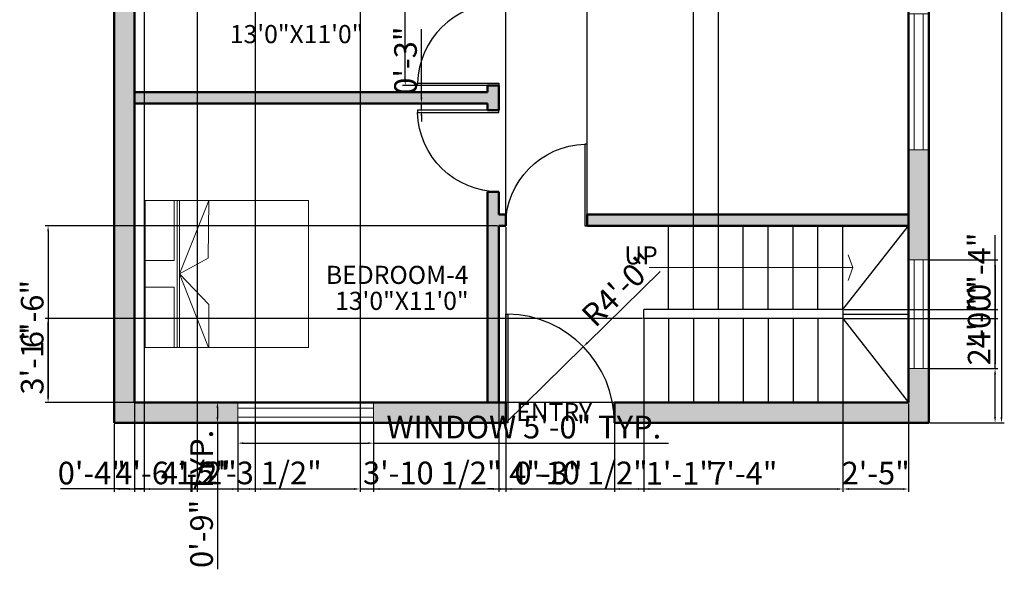
# Model space of a CAD drawing. Units: inches. Extents: x 2719 to 3167, y 1639 to 2327.
# Tile 1 of 4: x 2727 to 3162, y 1639 to 1881. Entities that reach past the tile are written whole.
import ezdxf

# ---------------------------------------------------------------- set-up
doc = ezdxf.new("R2010")
doc.units = ezdxf.units.IN
for name, color, linetype, lineweight in [('A-ANNO-DIMS', 121, 'Continuous', 18), ('A-ANNO-SYMB', 7, 'Continuous', 18), ('A-ANNO-TEXT', 121, 'Continuous', 18), ('A-AREA-IDEN', 121, 'Continuous', 18), ('A-DOOR', 50, 'Continuous', 25), ('A-FLOR-STRS', 7, 'Continuous', 25), ('A-FURN', 211, 'Continuous', 18), ('A-GLAZ', 191, 'Continuous', 18), ('A-WALL', 7, 'Continuous', 50)]:
    doc.layers.add(name, color=color, linetype=linetype, lineweight=lineweight)
doc.layers.add('A-WALL-PATT', color=251, linetype='Continuous', lineweight=13, true_color=0x636466)
doc.styles.get("Standard").update_dxf_attribs({"font": 'arial.ttf'})
doc.dimstyles.new('ISO-25', dxfattribs={"dimtxt": 10, "dimasz": 2.5, "dimexe": 1.25, "dimexo": 0.625, "dimtad": 1, "dimdec": 0, "dimlunit": 3, "dimtxsty": 'Standard', "dimcen": 2.5, "dimadec": 0, "dimazin": 0, "dimtfac": 1, "dimtdec": 0, "dimtmove": 0, "dimatfit": 3, "dimfxl": 1, "dimarcsym": 0})

# ---------------------------------------------------------------- blocks, each defined once
blk = doc.blocks.new('*D2')
at = {"layer": 'A-ANNO-DIMS', "color": 0, "lineweight": -2, "transparency": 16777216}
for p, q in [((3129.42, 2243.44), (3162.14, 2243.44)), ((3160.89, 2240.94), (3160.89, 1705.94)), ((3129.42, 1703.44), (3162.14, 1703.44))]:
    blk.add_line(p, q, dxfattribs=at)
at = {"layer": 'A-ANNO-DIMS', "color": 0, "transparency": 16777216}
for points in [[(3160.47, 2240.94), (3161.31, 2240.94), (3160.89, 2243.44)], [(3160.47, 1705.94), (3161.31, 1705.94), (3160.89, 1703.44)]]:
    blk.add_solid(points, dxfattribs=at)
at = {"layer": 'Defpoints', "color": 0, "transparency": 16777216}
for p in [(3128.8, 2243.44), (3128.8, 1703.44), (3160.89, 1703.44)]:
    blk.add_point(p, dxfattribs=at)
at = {"layer": 'A-ANNO-DIMS', "color": 0, "transparency": 16777216, "insert": (3155.18, 1973.44), "char_height": 10, "attachment_point": 5, "rotation": 90}
blk.add_mtext("45'", dxfattribs=at)
blk = doc.blocks.new('BED-DOUBLE')
for p, q in [((0, 57.96), (64.91, 57.96)), ((0, 56.96), (64.91, 56.96)), ((32.46, 56.96), (0, 44.1)), ((32.46, 56.96), (18.94, 44.05)), ((32.46, 56.96), (64.91, 44.04)), ((32.46, 56.96), (39.4, 44.29)), ((18.94, 44.05), (0, 44.05)), ((39.4, 44.29), (64.91, 44.04))]:
    blk.add_line(p, q)
for points in [[(0, 72.15), (64.91, 72.15), (64.91, 0), (0, 0)], [(0, 72.15), (26.55, 72.15), (26.55, 59.27), (0, 59.27)], [(38.37, 72.15), (64.91, 72.15), (64.91, 59.27), (38.37, 59.27)]]:
    blk.add_lwpolyline(points, close=True)
blk = doc.blocks.new('WIN-60IN')
for p, q in [((9, 60), (0, 60)), ((2.5, 60), (2.5, 0)), ((6.5, 60), (6.5, 0)), ((9, 0), (0, 0))]:
    blk.add_line(p, q)
blk = doc.blocks.new('DOOR-36IN-SWING')
for p, q in [((0, 0), (0, 1)), ((0, 1), (36, 1)), ((36, 0), (0, 0)), ((36, 1), (36, 0))]:
    blk.add_line(p, q)
blk.add_arc((35.99, 0), 36, 89.9779, 178.4083)
blk = doc.blocks.new('*D7')
at = {"layer": 'A-ANNO-DIMS', "color": 0, "lineweight": -2, "transparency": 16777216}
for p, q in [((2823.4, 1702.81), (2823.4, 1693.19)), ((2883.4, 1702.81), (2883.4, 1693.19)), ((2825.9, 1694.44), (2880.9, 1694.44)), ((2883.4, 1694.44), (3013.69, 1694.44))]:
    blk.add_line(p, q, dxfattribs=at)
at = {"layer": 'A-ANNO-DIMS', "color": 0, "transparency": 16777216}
for points in [[(2825.9, 1694.85), (2825.9, 1694.02), (2823.4, 1694.44)], [(2880.9, 1694.85), (2880.9, 1694.02), (2883.4, 1694.44)]]:
    blk.add_solid(points, dxfattribs=at)
at = {"layer": 'Defpoints', "color": 0, "transparency": 16777216}
for p in [(2823.4, 1703.44), (2883.4, 1703.44), (2883.4, 1694.44)]:
    blk.add_point(p, dxfattribs=at)
at = {"layer": 'A-ANNO-DIMS', "color": 0, "transparency": 16777216, "insert": (2949.79, 1700.24), "char_height": 10, "attachment_point": 5}
blk.add_mtext('WINDOW 5\'-0" TYP.', dxfattribs=at)
blk = doc.blocks.new('*D8')
at = {"layer": 'A-ANNO-DIMS', "color": 0, "lineweight": -2, "transparency": 16777216}
for p, q in [((2822.77, 1712.44), (2813.15, 1712.44)), ((2814.4, 1709.94), (2814.4, 1705.94)), ((2822.77, 1703.44), (2813.15, 1703.44)), ((2814.4, 1703.44), (2814.4, 1638.73))]:
    blk.add_line(p, q, dxfattribs=at)
at = {"layer": 'A-ANNO-DIMS', "color": 0, "transparency": 16777216}
for points in [[(2813.98, 1709.94), (2814.82, 1709.94), (2814.4, 1712.44)], [(2813.98, 1705.94), (2814.82, 1705.94), (2814.4, 1703.44)]]:
    blk.add_solid(points, dxfattribs=at)
at = {"layer": 'Defpoints', "color": 0, "transparency": 16777216}
for p in [(2823.4, 1712.44), (2814.4, 1703.44), (2823.4, 1703.44)]:
    blk.add_point(p, dxfattribs=at)
at = {"layer": 'A-ANNO-DIMS', "color": 0, "transparency": 16777216, "insert": (2808.67, 1669.83), "char_height": 10, "attachment_point": 5, "rotation": 90}
blk.add_mtext('0\'-9" TYP.', dxfattribs=at)
blk = doc.blocks.new('*D11')
at = {"layer": 'A-ANNO-DIMS', "color": 0, "lineweight": -2, "transparency": 16777216}
for p, q in [((2897.39, 1888.44), (2897.39, 2011.64)), ((2902.17, 1888.44), (2896.14, 1888.44)), ((2897.39, 1854.94), (2897.39, 1885.94)), ((2902.17, 1852.44), (2896.14, 1852.44))]:
    blk.add_line(p, q, dxfattribs=at)
at = {"layer": 'A-ANNO-DIMS', "color": 0, "transparency": 16777216}
for points in [[(2896.98, 1885.94), (2897.81, 1885.94), (2897.39, 1888.44)], [(2896.98, 1854.94), (2897.81, 1854.94), (2897.39, 1852.44)]]:
    blk.add_solid(points, dxfattribs=at)
at = {"layer": 'Defpoints', "color": 0, "transparency": 16777216}
for p in [(2897.39, 1888.44), (2902.8, 1888.44), (2902.8, 1852.44)]:
    blk.add_point(p, dxfattribs=at)
at = {"layer": 'A-ANNO-DIMS', "color": 0, "transparency": 16777216, "insert": (2891.59, 1951.29), "char_height": 10, "attachment_point": 5, "rotation": 90}
blk.add_mtext('DOOR A 3\'-0" TYP.', dxfattribs=at)
blk = doc.blocks.new('*D15')
at = {"layer": 'A-ANNO-DIMS', "color": 0, "lineweight": -2, "transparency": 16777216}
for p, q in [((2768.8, 1702.81), (2768.8, 1672.94)), ((2823.4, 1702.81), (2823.4, 1672.94)), ((2771.3, 1674.19), (2820.9, 1674.19))]:
    blk.add_line(p, q, dxfattribs=at)
at = {"layer": 'A-ANNO-DIMS', "color": 0, "transparency": 16777216}
for points in [[(2771.3, 1674.6), (2771.3, 1673.77), (2768.8, 1674.19)], [(2820.9, 1674.6), (2820.9, 1673.77), (2823.4, 1674.19)]]:
    blk.add_solid(points, dxfattribs=at)
at = {"layer": 'Defpoints', "color": 0, "transparency": 16777216}
for p in [(2768.8, 1703.44), (2823.4, 1703.44), (2823.4, 1674.19)]:
    blk.add_point(p, dxfattribs=at)
at = {"layer": 'A-ANNO-DIMS', "color": 0, "transparency": 16777216, "insert": (2796.1, 1679.98), "char_height": 10, "attachment_point": 5}
blk.add_mtext('4\'-6 1/2"', dxfattribs=at)
blk = doc.blocks.new('*D16')
at = {"layer": 'A-ANNO-DIMS', "color": 0, "lineweight": -2, "transparency": 16777216}
for p, q in [((2883.4, 1702.81), (2883.4, 1672.94)), ((2941.8, 1702.81), (2941.8, 1672.94)), ((2885.9, 1674.19), (2939.3, 1674.19)), ((2941.8, 1674.19), (3003.6, 1674.19))]:
    blk.add_line(p, q, dxfattribs=at)
at = {"layer": 'A-ANNO-DIMS', "color": 0, "transparency": 16777216}
for points in [[(2885.9, 1674.6), (2885.9, 1673.77), (2883.4, 1674.19)], [(2939.3, 1674.6), (2939.3, 1673.77), (2941.8, 1674.19)]]:
    blk.add_solid(points, dxfattribs=at)
at = {"layer": 'Defpoints', "color": 0, "transparency": 16777216}
for p in [(2883.4, 1703.44), (2941.8, 1703.44), (2941.8, 1674.19)]:
    blk.add_point(p, dxfattribs=at)
at = {"layer": 'A-ANNO-DIMS', "color": 0, "transparency": 16777216, "insert": (2973.95, 1679.98), "char_height": 10, "attachment_point": 5}
blk.add_mtext('4\'-10 1/2"', dxfattribs=at)
blk = doc.blocks.new('*D26')
at = {"layer": 'A-ANNO-DIMS', "color": 0, "lineweight": -2, "transparency": 16777216}
for p, q in [((3158.05, 1727.34), (3158.05, 1757.84)), ((3129.42, 1727.34), (3159.3, 1727.34)), ((3158.05, 1705.94), (3158.05, 1724.84)), ((3129.42, 1703.44), (3159.3, 1703.44))]:
    blk.add_line(p, q, dxfattribs=at)
at = {"layer": 'A-ANNO-DIMS', "color": 0, "transparency": 16777216}
for points in [[(3157.63, 1724.84), (3158.46, 1724.84), (3158.05, 1727.34)], [(3157.63, 1705.94), (3158.46, 1705.94), (3158.05, 1703.44)]]:
    blk.add_solid(points, dxfattribs=at)
at = {"layer": 'Defpoints', "color": 0, "transparency": 16777216}
for p in [(3128.8, 1727.34), (3158.05, 1727.34), (3128.8, 1703.44)]:
    blk.add_point(p, dxfattribs=at)
at = {"layer": 'A-ANNO-DIMS', "color": 0, "transparency": 16777216, "insert": (3152.32, 1743.84), "char_height": 10, "attachment_point": 5, "rotation": 90}
blk.add_mtext('2\'-0"', dxfattribs=at)
blk = doc.blocks.new('*D27')
at = {"layer": 'A-ANNO-DIMS', "color": 0, "lineweight": -2, "transparency": 16777216}
for p, q in [((3129.42, 1775.34), (3159.3, 1775.34)), ((3158.05, 1772.84), (3158.05, 1729.84)), ((3129.42, 1727.34), (3159.3, 1727.34))]:
    blk.add_line(p, q, dxfattribs=at)
at = {"layer": 'A-ANNO-DIMS', "color": 0, "transparency": 16777216}
for points in [[(3157.63, 1772.84), (3158.46, 1772.84), (3158.05, 1775.34)], [(3157.63, 1729.84), (3158.46, 1729.84), (3158.05, 1727.34)]]:
    blk.add_solid(points, dxfattribs=at)
at = {"layer": 'Defpoints', "color": 0, "transparency": 16777216}
for p in [(3128.8, 1775.34), (3128.8, 1727.34), (3158.05, 1727.34)]:
    blk.add_point(p, dxfattribs=at)
at = {"layer": 'A-ANNO-DIMS', "color": 0, "transparency": 16777216, "insert": (3152.32, 1751.34), "char_height": 10, "attachment_point": 5, "rotation": 90}
blk.add_mtext('4\'-0"', dxfattribs=at)
blk = doc.blocks.new('*D31')
at = {"layer": 'A-ANNO-DIMS', "color": 0, "lineweight": -2, "transparency": 16777216}
for p, q in [((2777.8, 1985.81), (2777.8, 1672.94)), ((2805.5, 1985.81), (2805.5, 1672.94)), ((2780.3, 1674.19), (2803, 1674.19)), ((2805.5, 1674.19), (2859.31, 1674.19))]:
    blk.add_line(p, q, dxfattribs=at)
at = {"layer": 'A-ANNO-DIMS', "color": 0, "transparency": 16777216}
for points in [[(2780.3, 1674.6), (2780.3, 1673.77), (2777.8, 1674.19)], [(2803, 1674.6), (2803, 1673.77), (2805.5, 1674.19)]]:
    blk.add_solid(points, dxfattribs=at)
at = {"layer": 'Defpoints', "color": 0, "transparency": 16777216}
for p in [(2777.8, 1986.44), (2805.5, 1986.44), (2805.5, 1674.19)]:
    blk.add_point(p, dxfattribs=at)
at = {"layer": 'A-ANNO-DIMS', "color": 0, "transparency": 16777216, "insert": (2833.65, 1679.99), "char_height": 10, "attachment_point": 5}
blk.add_mtext('2\'-3 1/2"', dxfattribs=at)
blk = doc.blocks.new('*D36')
at = {"layer": 'A-ANNO-DIMS', "color": 0, "lineweight": -2, "transparency": 16777216}
for p, q in [((2782.04, 2006.33), (2782.04, 1672.94)), ((2777.8, 1985.81), (2777.8, 1672.94)), ((2775.3, 1674.19), (2744.96, 1674.19)), ((2782.04, 1674.19), (2777.8, 1674.19)), ((2784.54, 1674.19), (2787.04, 1674.19))]:
    blk.add_line(p, q, dxfattribs=at)
at = {"layer": 'A-ANNO-DIMS', "color": 0, "transparency": 16777216}
for points in [[(2775.3, 1674.6), (2775.3, 1673.77), (2777.8, 1674.19)], [(2784.54, 1674.6), (2784.54, 1673.77), (2782.04, 1674.19)]]:
    blk.add_solid(points, dxfattribs=at)
at = {"layer": 'Defpoints', "color": 0, "transparency": 16777216}
for p in [(2782.04, 2006.96), (2777.8, 1986.44), (2777.8, 1674.19)]:
    blk.add_point(p, dxfattribs=at)
at = {"layer": 'A-ANNO-DIMS', "color": 0, "transparency": 16777216, "insert": (2758.88, 1679.92), "char_height": 10, "attachment_point": 5}
blk.add_mtext('0\'-4"', dxfattribs=at)
blk = doc.blocks.new('*D37')
at = {"layer": 'A-ANNO-DIMS', "color": 0, "lineweight": -2, "transparency": 16777216}
for p, q in [((2831.04, 2061.64), (2831.04, 1672.94)), ((2877.4, 2061.64), (2877.4, 1672.94)), ((2833.54, 1674.19), (2874.9, 1674.19)), ((2877.4, 1674.19), (2938.79, 1674.19))]:
    blk.add_line(p, q, dxfattribs=at)
at = {"layer": 'A-ANNO-DIMS', "color": 0, "transparency": 16777216}
for points in [[(2833.54, 1674.6), (2833.54, 1673.77), (2831.04, 1674.19)], [(2874.9, 1674.6), (2874.9, 1673.77), (2877.4, 1674.19)]]:
    blk.add_solid(points, dxfattribs=at)
at = {"layer": 'Defpoints', "color": 0, "transparency": 16777216}
for p in [(2831.04, 2062.26), (2877.4, 2062.26), (2877.4, 1674.19)]:
    blk.add_point(p, dxfattribs=at)
at = {"layer": 'A-ANNO-DIMS', "color": 0, "transparency": 16777216, "insert": (2909.34, 1679.99), "char_height": 10, "attachment_point": 5}
blk.add_mtext('3\'-10 1/2"', dxfattribs=at)
blk = doc.blocks.new('*D39')
at = {"layer": 'A-ANNO-DIMS', "color": 0, "lineweight": -2, "transparency": 16777216}
for p, q in [((2777.8, 2084.81), (2777.8, 1672.94)), ((2831.04, 2061.64), (2831.04, 1672.94)), ((2780.3, 1674.19), (2828.54, 1674.19))]:
    blk.add_line(p, q, dxfattribs=at)
at = {"layer": 'A-ANNO-DIMS', "color": 0, "transparency": 16777216}
for points in [[(2780.3, 1674.6), (2780.3, 1673.77), (2777.8, 1674.19)], [(2828.54, 1674.6), (2828.54, 1673.77), (2831.04, 1674.19)]]:
    blk.add_solid(points, dxfattribs=at)
at = {"layer": 'Defpoints', "color": 0, "transparency": 16777216}
for p in [(2777.8, 2085.44), (2831.04, 2062.26), (2831.04, 1674.19)]:
    blk.add_point(p, dxfattribs=at)
at = {"layer": 'A-ANNO-DIMS', "color": 0, "transparency": 16777216, "insert": (2804.42, 1679.9), "char_height": 10, "attachment_point": 5}
blk.add_mtext('4\'-5"', dxfattribs=at)
blk = doc.blocks.new('*D41')
at = {"layer": 'A-ANNO-DIMS', "color": 0, "lineweight": -2, "transparency": 16777216}
for p, q in [((3002.8, 1711.81), (3002.8, 1672.94)), ((3090.8, 1711.81), (3090.8, 1672.94)), ((3005.3, 1674.19), (3088.3, 1674.19))]:
    blk.add_line(p, q, dxfattribs=at)
at = {"layer": 'A-ANNO-DIMS', "color": 0, "transparency": 16777216}
for points in [[(3005.3, 1674.6), (3005.3, 1673.77), (3002.8, 1674.19)], [(3088.3, 1674.6), (3088.3, 1673.77), (3090.8, 1674.19)]]:
    blk.add_solid(points, dxfattribs=at)
at = {"layer": 'Defpoints', "color": 0, "transparency": 16777216}
for p in [(3002.8, 1712.44), (3090.8, 1712.44), (3090.8, 1674.19)]:
    blk.add_point(p, dxfattribs=at)
at = {"layer": 'A-ANNO-DIMS', "color": 0, "transparency": 16777216, "insert": (3046.8, 1679.81), "char_height": 10, "attachment_point": 5}
blk.add_mtext('7\'-4"', dxfattribs=at)
blk = doc.blocks.new('*D42')
at = {"layer": 'A-ANNO-DIMS', "color": 0, "lineweight": -2, "transparency": 16777216}
for p, q in [((3090.8, 1711.81), (3090.8, 1672.94)), ((3119.8, 1711.81), (3119.8, 1672.94)), ((3093.3, 1674.19), (3117.3, 1674.19))]:
    blk.add_line(p, q, dxfattribs=at)
at = {"layer": 'A-ANNO-DIMS', "color": 0, "transparency": 16777216}
for points in [[(3093.3, 1674.6), (3093.3, 1673.77), (3090.8, 1674.19)], [(3117.3, 1674.6), (3117.3, 1673.77), (3119.8, 1674.19)]]:
    blk.add_solid(points, dxfattribs=at)
at = {"layer": 'Defpoints', "color": 0, "transparency": 16777216}
for p in [(3090.8, 1712.44), (3119.8, 1712.44), (3119.8, 1674.19)]:
    blk.add_point(p, dxfattribs=at)
at = {"layer": 'A-ANNO-DIMS', "color": 0, "transparency": 16777216, "insert": (3105.3, 1679.92), "char_height": 10, "attachment_point": 5}
blk.add_mtext('2\'-5"', dxfattribs=at)
blk = doc.blocks.new('*D43')
at = {"layer": 'A-ANNO-DIMS', "color": 0, "lineweight": -2, "transparency": 16777216}
for p, q in [((2989.8, 1711.81), (2989.8, 1672.94)), ((3002.8, 1711.81), (3002.8, 1672.94)), ((2992.3, 1674.19), (3000.3, 1674.19)), ((3002.8, 1674.19), (3032.19, 1674.19))]:
    blk.add_line(p, q, dxfattribs=at)
at = {"layer": 'A-ANNO-DIMS', "color": 0, "transparency": 16777216}
for points in [[(2992.3, 1674.6), (2992.3, 1673.77), (2989.8, 1674.19)], [(3000.3, 1674.6), (3000.3, 1673.77), (3002.8, 1674.19)]]:
    blk.add_solid(points, dxfattribs=at)
at = {"layer": 'Defpoints', "color": 0, "transparency": 16777216}
for p in [(2989.8, 1712.44), (3002.8, 1712.44), (3002.8, 1674.19)]:
    blk.add_point(p, dxfattribs=at)
at = {"layer": 'A-ANNO-DIMS', "color": 0, "transparency": 16777216, "insert": (3018.74, 1679.83), "char_height": 10, "attachment_point": 5}
blk.add_mtext('1\'-1"', dxfattribs=at)
blk = doc.blocks.new('*D44')
at = {"layer": 'A-ANNO-DIMS', "color": 0, "lineweight": -2, "transparency": 16777216}
for p, q in [((3002.17, 1749.44), (2738.3, 1749.44)), ((2739.55, 1714.94), (2739.55, 1746.94)), ((3002.17, 1712.44), (2738.3, 1712.44))]:
    blk.add_line(p, q, dxfattribs=at)
at = {"layer": 'A-ANNO-DIMS', "color": 0, "transparency": 16777216}
for points in [[(2739.13, 1746.94), (2739.96, 1746.94), (2739.55, 1749.44)], [(2739.13, 1714.94), (2739.96, 1714.94), (2739.55, 1712.44)]]:
    blk.add_solid(points, dxfattribs=at)
at = {"layer": 'Defpoints', "color": 0, "transparency": 16777216}
for p in [(2739.55, 1749.44), (3002.8, 1749.44), (3002.8, 1712.44)]:
    blk.add_point(p, dxfattribs=at)
at = {"layer": 'A-ANNO-DIMS', "color": 0, "transparency": 16777216, "insert": (2733.81, 1730.94), "char_height": 10, "attachment_point": 5, "rotation": 90}
blk.add_mtext('3\'-1"', dxfattribs=at)
blk = doc.blocks.new('*D45')
at = {"layer": 'A-ANNO-DIMS', "color": 0, "lineweight": -2, "transparency": 16777216}
for p, q in [((3158.05, 1755.94), (3158.05, 1786.27)), ((3091.42, 1753.44), (3159.3, 1753.44)), ((3091.42, 1749.44), (3159.3, 1749.44)), ((3158.05, 1749.44), (3158.05, 1753.44)), ((3158.05, 1746.94), (3158.05, 1744.44))]:
    blk.add_line(p, q, dxfattribs=at)
at = {"layer": 'A-ANNO-DIMS', "color": 0, "transparency": 16777216}
for points in [[(3157.63, 1755.94), (3158.46, 1755.94), (3158.05, 1753.44)], [(3157.63, 1746.94), (3158.46, 1746.94), (3158.05, 1749.44)]]:
    blk.add_solid(points, dxfattribs=at)
at = {"layer": 'Defpoints', "color": 0, "transparency": 16777216}
for p in [(3090.8, 1753.44), (3090.8, 1749.44), (3158.05, 1753.44)]:
    blk.add_point(p, dxfattribs=at)
at = {"layer": 'A-ANNO-DIMS', "color": 0, "transparency": 16777216, "insert": (3152.32, 1772.35), "char_height": 10, "attachment_point": 5, "rotation": 90}
blk.add_mtext('0\'-4"', dxfattribs=at)
blk = doc.blocks.new('*D46')
at = {"layer": 'A-ANNO-DIMS', "color": 0, "lineweight": -2, "transparency": 16777216}
for p, q in [((3024.8, 1791.06), (3024.8, 2273.94)), ((3027.3, 2272.69), (3033.3, 2272.69)), ((3035.8, 1791.06), (3035.8, 2273.94)), ((3035.8, 2272.69), (3073.9, 2272.69))]:
    blk.add_line(p, q, dxfattribs=at)
at = {"layer": 'A-ANNO-DIMS', "color": 0, "transparency": 16777216}
for points in [[(3027.3, 2273.1), (3027.3, 2272.27), (3024.8, 2272.69)], [(3033.3, 2273.1), (3033.3, 2272.27), (3035.8, 2272.69)]]:
    blk.add_solid(points, dxfattribs=at)
at = {"layer": 'Defpoints', "color": 0, "transparency": 16777216}
for p in [(3035.8, 2272.69), (3024.8, 1790.44), (3035.8, 1790.44)]:
    blk.add_point(p, dxfattribs=at)
at = {"layer": 'A-ANNO-DIMS', "color": 0, "transparency": 16777216, "insert": (3056.1, 2278.42), "char_height": 10, "attachment_point": 5}
blk.add_mtext('0\'-11"', dxfattribs=at)
blk = doc.blocks.new('*D47')
at = {"layer": 'A-ANNO-DIMS', "color": 0, "lineweight": -2, "transparency": 16777216}
for p, q in [((2938.17, 1790.44), (2738.3, 1790.44)), ((2739.55, 1787.94), (2739.55, 1714.94)), ((2938.17, 1712.44), (2738.3, 1712.44))]:
    blk.add_line(p, q, dxfattribs=at)
at = {"layer": 'A-ANNO-DIMS', "color": 0, "transparency": 16777216}
for points in [[(2739.13, 1787.94), (2739.96, 1787.94), (2739.55, 1790.44)], [(2739.13, 1714.94), (2739.96, 1714.94), (2739.55, 1712.44)]]:
    blk.add_solid(points, dxfattribs=at)
at = {"layer": 'Defpoints', "color": 0, "transparency": 16777216}
for p in [(2938.8, 1790.44), (2739.55, 1712.44), (2938.8, 1712.44)]:
    blk.add_point(p, dxfattribs=at)
at = {"layer": 'A-ANNO-DIMS', "color": 0, "transparency": 16777216, "insert": (2733.82, 1751.44), "char_height": 10, "attachment_point": 5, "rotation": 90}
blk.add_mtext('6\'-6"', dxfattribs=at)
blk = doc.blocks.new('*D48')
at = {"layer": 'A-ANNO-DIMS', "color": 0, "lineweight": -2, "transparency": 16777216}
for p, q in [((2941.8, 1796.06), (2941.8, 2273.94)), ((2944.3, 2272.69), (2975.3, 2272.69)), ((2977.8, 1796.06), (2977.8, 2273.94))]:
    blk.add_line(p, q, dxfattribs=at)
at = {"layer": 'A-ANNO-DIMS', "color": 0, "transparency": 16777216}
for points in [[(2944.3, 2273.1), (2944.3, 2272.27), (2941.8, 2272.69)], [(2975.3, 2273.1), (2975.3, 2272.27), (2977.8, 2272.69)]]:
    blk.add_solid(points, dxfattribs=at)
at = {"layer": 'Defpoints', "color": 0, "transparency": 16777216}
for p in [(2977.8, 2272.69), (2941.8, 1795.44), (2977.8, 1795.44)]:
    blk.add_point(p, dxfattribs=at)
at = {"layer": 'A-ANNO-DIMS', "color": 0, "transparency": 16777216, "insert": (2959.8, 2278.42), "char_height": 10, "attachment_point": 5}
blk.add_mtext('3\'-0"', dxfattribs=at)
blk = doc.blocks.new('*D49')
at = {"layer": 'A-ANNO-DIMS', "color": 0, "lineweight": -2, "transparency": 16777216}
for p, q in [((2938.8, 1789.81), (2938.8, 1672.94)), ((2941.8, 1789.81), (2941.8, 1672.94)), ((2936.3, 1674.19), (2933.8, 1674.19)), ((2938.8, 1674.19), (2941.8, 1674.19)), ((2944.3, 1674.19), (2974.63, 1674.19))]:
    blk.add_line(p, q, dxfattribs=at)
at = {"layer": 'A-ANNO-DIMS', "color": 0, "transparency": 16777216}
for points in [[(2936.3, 1674.6), (2936.3, 1673.77), (2938.8, 1674.19)], [(2944.3, 1674.6), (2944.3, 1673.77), (2941.8, 1674.19)]]:
    blk.add_solid(points, dxfattribs=at)
at = {"layer": 'Defpoints', "color": 0, "transparency": 16777216}
for p in [(2938.8, 1790.44), (2941.8, 1790.44), (2941.8, 1674.19)]:
    blk.add_point(p, dxfattribs=at)
at = {"layer": 'A-ANNO-DIMS', "color": 0, "transparency": 16777216, "insert": (2960.71, 1679.92), "char_height": 10, "attachment_point": 5}
blk.add_mtext('0\'-3"', dxfattribs=at)
blk = doc.blocks.new('*D50')
at = {"layer": 'A-ANNO-DIMS', "color": 0, "lineweight": -2, "transparency": 16777216}
for p, q in [((2904.55, 1846.94), (2904.55, 1877.27)), ((2933.17, 1844.44), (2903.3, 1844.44)), ((2933.17, 1841.44), (2903.3, 1841.44)), ((2904.55, 1841.44), (2904.55, 1844.44)), ((2904.55, 1838.94), (2904.55, 1836.44))]:
    blk.add_line(p, q, dxfattribs=at)
at = {"layer": 'A-ANNO-DIMS', "color": 0, "transparency": 16777216}
for points in [[(2904.13, 1846.94), (2904.96, 1846.94), (2904.55, 1844.44)], [(2904.13, 1838.94), (2904.96, 1838.94), (2904.55, 1841.44)]]:
    blk.add_solid(points, dxfattribs=at)
at = {"layer": 'Defpoints', "color": 0, "transparency": 16777216}
for p in [(2904.55, 1844.44), (2933.8, 1844.44), (2933.8, 1841.44)]:
    blk.add_point(p, dxfattribs=at)
at = {"layer": 'A-ANNO-DIMS', "color": 0, "transparency": 16777216, "insert": (2898.81, 1863.35), "char_height": 10, "attachment_point": 5, "rotation": 90}
blk.add_mtext('0\'-3"', dxfattribs=at)
blk = doc.blocks.new('*D53')
at = {"layer": 'A-ANNO-DIMS', "color": 0, "lineweight": -2, "transparency": 16777216}
for p, q in [((3010.03, 1770.26), (2977.88, 1738.78)), ((2941.8, 1703.45), (2976.09, 1737.03))]:
    blk.add_line(p, q, dxfattribs=at)
at = {"layer": 'A-ANNO-DIMS', "color": 0, "transparency": 16777216}
blk.add_solid([(2977.59, 1739.08), (2978.17, 1738.48), (2976.09, 1737.03)], dxfattribs=at)
at = {"layer": 'Defpoints', "color": 0, "transparency": 16777216}
for p in [(2976.09, 1737.03), (2941.8, 1703.45)]:
    blk.add_point(p, dxfattribs=at)
at = {"layer": 'A-ANNO-DIMS', "color": 0, "transparency": 16777216, "insert": (2992.66, 1761.27), "char_height": 10, "attachment_point": 5, "rotation": 44.3967}
blk.add_mtext('R4\'-0"', dxfattribs=at)

msp = doc.modelspace()

# ---------------------------------------------------------------- hatches: boundary and pattern name
at = {"layer": 'A-WALL-PATT'}
h = msp.add_hatch(color=256, dxfattribs=at)
h.dxf.hatch_style = 1
h.paths.add_polyline_path([(2777.8, 1884.83), (2768.8, 1884.83), (2768.8, 1703.44), (2823.4, 1703.44), (2823.4, 1712.44), (2777.8, 1712.44)])
h = msp.add_hatch(color=256, dxfattribs=at)
h.dxf.hatch_style = 1
h.paths.add_polyline_path([(2938.8, 1852.44), (2933.8, 1852.44), (2933.8, 1849.44), (2777.8, 1849.44), (2777.8, 1844.44), (2933.8, 1844.44), (2933.8, 1841.44), (2938.8, 1841.44)])
h = msp.add_hatch(color=256, dxfattribs=at)
h.dxf.hatch_style = 1
h.paths.add_polyline_path([(3128.8, 1823.95), (3119.8, 1823.95), (3119.8, 1775.34), (3128.8, 1775.34)])
h = msp.add_hatch(color=256, dxfattribs=at)
h.dxf.hatch_style = 1
h.paths.add_polyline_path([(2938.8, 1790.44), (2941.8, 1790.44), (2941.8, 1795.44), (2938.8, 1795.44), (2938.8, 1805.44), (2933.8, 1805.44), (2933.8, 1712.44), (2938.8, 1712.44)])
h = msp.add_hatch(color=256, dxfattribs=at)
h.dxf.hatch_style = 1
h.paths.add_polyline_path([(3119.8, 1795.44), (2977.8, 1795.44), (2977.8, 1790.44), (3119.8, 1790.44)])
h = msp.add_hatch(color=256, dxfattribs=at)
h.dxf.hatch_style = 1
h.paths.add_polyline_path([(3128.8, 1727.34), (3119.8, 1727.34), (3119.8, 1712.44), (2989.8, 1712.44), (2989.8, 1703.44), (3128.8, 1703.44)])
h = msp.add_hatch(color=256, dxfattribs=at)
h.dxf.hatch_style = 1
h.paths.add_polyline_path([(2941.8, 1712.44), (2883.4, 1712.44), (2883.4, 1703.44), (2941.8, 1703.44)])

# ---------------------------------------------------------------- linework, layer by layer
at = {"layer": 'A-ANNO-SYMB'}
for p, q in [((3095.16, 1771.94), (3093.11, 1777.58)), ((3005.17, 1771.94), (3095.16, 1771.94)), ((3095.16, 1771.94), (3093.11, 1766.3))]:
    msp.add_line(p, q, dxfattribs=at)
at = {"layer": 'A-DOOR'}
for p, q in [((2941.8, 1703.44), (2941.8, 1751.44)), ((2941.8, 1751.44), (2942.8, 1751.44)), ((2942.8, 1751.44), (2942.8, 1703.44)), ((2942.8, 1703.44), (2941.8, 1703.44))]:
    msp.add_line(p, q, dxfattribs=at)
msp.add_arc((2941.8, 1703.45), 48, 359.9876, 88.8063, dxfattribs=at)
at = {"layer": 'A-FLOR-STRS'}
for p, q in [((3013.8, 1753.44), (3013.8, 1790.44)), ((3024.8, 1753.44), (3024.8, 1790.44)), ((3035.8, 1753.44), (3035.8, 1790.44)), ((3046.8, 1753.44), (3046.8, 1790.44)), ((3057.8, 1753.44), (3057.8, 1790.44)), ((3068.8, 1753.44), (3068.8, 1790.44)), ((3079.8, 1753.44), (3079.8, 1790.44)), ((3090.8, 1753.44), (3090.8, 1790.44)), ((3090.8, 1753.44), (3119.8, 1790.44)), ((3090.8, 1753.44), (3002.8, 1753.44)), ((3002.8, 1749.44), (3002.8, 1753.44)), ((3090.8, 1749.44), (3002.8, 1749.44)), ((3002.8, 1749.44), (3002.8, 1712.44)), ((3013.8, 1749.44), (3013.8, 1712.44)), ((3024.8, 1749.44), (3024.8, 1712.44)), ((3035.8, 1749.44), (3035.8, 1712.44)), ((3046.8, 1749.44), (3046.8, 1712.44)), ((3057.8, 1749.44), (3057.8, 1712.44)), ((3068.8, 1749.44), (3068.8, 1712.44)), ((3079.8, 1749.44), (3079.8, 1712.44)), ((3090.8, 1753.44), (3090.8, 1749.44)), ((3090.8, 1751.44), (3119.8, 1751.44)), ((3090.8, 1749.44), (3090.8, 1712.44)), ((3090.8, 1749.44), (3119.8, 1712.44))]:
    msp.add_line(p, q, dxfattribs=at)
at = {"layer": 'A-GLAZ'}
for p, q in [((3119.8, 1775.34), (3128.8, 1775.34)), ((3122.3, 1775.34), (3122.3, 1727.34)), ((3126.3, 1775.34), (3126.3, 1727.34)), ((3119.8, 1727.34), (3128.8, 1727.34))]:
    msp.add_line(p, q, dxfattribs=at)
at = {"layer": 'A-WALL'}
for p, q in [((2777.8, 1712.44), (2777.8, 2234.44)), ((3119.8, 2234.44), (3119.8, 1712.44)), ((2777.8, 1849.44), (2933.8, 1849.44)), ((2933.8, 1852.44), (2938.8, 1852.44)), ((2933.8, 1849.44), (2933.8, 1852.44)), ((2938.8, 1841.44), (2938.8, 1852.44)), ((2777.8, 1844.44), (2933.8, 1844.44)), ((2933.8, 1841.44), (2933.8, 1844.44)), ((2933.8, 1841.44), (2938.8, 1841.44)), ((2933.8, 1712.44), (2933.8, 1805.44)), ((2933.8, 1805.44), (2938.8, 1805.44)), ((2938.8, 1795.44), (2938.8, 1805.44)), ((2941.8, 1795.44), (2938.8, 1795.44)), ((2941.8, 1795.44), (2941.8, 1790.44)), ((3119.8, 1795.44), (2977.8, 1795.44)), ((2977.8, 1795.44), (2977.8, 1790.44)), ((2938.8, 1712.44), (2938.8, 1790.44)), ((2941.8, 1790.44), (2938.8, 1790.44)), ((3119.8, 1790.44), (2977.8, 1790.44)), ((2941.8, 1712.44), (2777.8, 1712.44)), ((2941.8, 1712.44), (2941.8, 1703.44)), ((3119.8, 1712.44), (2989.8, 1712.44)), ((2989.8, 1712.44), (2989.8, 1703.44))]:
    msp.add_line(p, q, dxfattribs=at)
msp.add_lwpolyline([(2941.8, 1703.44), (2768.8, 1703.44), (2768.8, 2243.44), (3128.8, 2243.44), (3128.8, 1703.44), (2989.8, 1703.44)], dxfattribs=at)

# ---------------------------------------------------------------- block references
at = {"layer": 'A-DOOR'}
msp.add_blockref('DOOR-36IN-SWING', (2902.8, 1852.44), dxfattribs=at)
at = {"layer": 'A-DOOR', "extrusion": (0, 0, -1), "zscale": -1}
for p, rotation in [((-2902.8, 1841.44), 180), ((-2977.8, 1826.44), 270.0000000000013)]:
    msp.add_blockref('DOOR-36IN-SWING', p, dxfattribs=dict(at, rotation=rotation))
at = {"layer": 'A-FURN', "rotation": 89.99999999999875}
msp.add_blockref('BED-DOUBLE', (2854.59, 1736.74), dxfattribs=at)
at = {"layer": 'A-GLAZ'}
msp.add_blockref('WIN-60IN', (3119.8, 1823.95), dxfattribs=at)
at = {"layer": 'A-GLAZ', "rotation": 270}
msp.add_blockref('WIN-60IN', (2823.4, 1712.44), dxfattribs=at)

# ---------------------------------------------------------------- texts
at = {"layer": 'A-ANNO-TEXT'}
for tag, p in [('UP', (2994.2, 1773.35)), ('ENTRY', (2946.43, 1704.18))]:
    msp.add_attdef(tag, p, '', height=8, dxfattribs=at)
at = {"layer": 'A-AREA-IDEN'}
for tag, p in [('13\'0"X11\'0"', (2819.88, 1871.07)), ('BEDROOM-4', (2862.35, 1764.74)), ('13\'0"X11\'0"', (2866.38, 1753.28))]:
    msp.add_attdef(tag, p, '', height=8, dxfattribs=at)

# ---------------------------------------------------------------- dimensions: what is measured, and where the dimension line sits
at = {"layer": 'A-ANNO-DIMS'}
for base, p1, p2, picture, middle in [((2977.8, 2272.69), (2941.8, 1795.44), (2977.8, 1795.44), '*D48', (2959.8, 2278.42)), ((3035.8, 2272.69), (3024.8, 1790.44), (3035.8, 1790.44), '*D46', (3056.1, 2278.42)), ((2831.04, 1674.19), (2777.8, 2085.44), (2831.04, 2062.26), '*D39', (2804.42, 1679.9)), ((2877.4, 1674.19), (2831.04, 2062.26), (2877.4, 2062.26), '*D37', (2909.34, 1679.99)), ((2777.8, 1674.19), (2782.04, 2006.96), (2777.8, 1986.44), '*D36', (2758.88, 1679.92)), ((2805.5, 1674.19), (2777.8, 1986.44), (2805.5, 1986.44), '*D31', (2833.65, 1679.99)), ((2941.8, 1674.19), (2938.8, 1790.44), (2941.8, 1790.44), '*D49', (2960.71, 1679.92)), ((3002.8, 1674.19), (2989.8, 1712.44), (3002.8, 1712.44), '*D43', (3018.74, 1679.83)), ((3090.8, 1674.19), (3002.8, 1712.44), (3090.8, 1712.44), '*D41', (3046.8, 1679.81)), ((3119.8, 1674.19), (3090.8, 1712.44), (3119.8, 1712.44), '*D42', (3105.3, 1679.92)), ((2823.4, 1674.19), (2768.8, 1703.44), (2823.4, 1703.44), '*D15', (2796.1, 1679.98)), ((2941.8, 1674.19), (2883.4, 1703.44), (2941.8, 1703.44), '*D16', (2973.95, 1679.98))]:
    dim = msp.add_linear_dim(base=base, p1=p1, p2=p2, dimstyle='ISO-25', override={"dimdec": 1, "dimlfac": 1, "dimrnd": 0, "dimzin": 1, "dimdsep": 46, "dimlunit": 4, "dimfrac": 2}, dxfattribs=at)
    dim.commit()
    dim.dimension.update_dxf_attribs({"geometry": picture, "text_midpoint": middle})
for base, p1, p2, override, picture, middle in [((3160.89, 1703.44), (3128.8, 2243.44), (3128.8, 1703.44), {"dimclrd": 0, "dimclre": 0, "dimclrt": 0}, '*D2', (3155.18, 1973.44)), ((2904.55, 1844.44), (2933.8, 1841.44), (2933.8, 1844.44), {"dimdec": 1, "dimlfac": 1, "dimrnd": 0, "dimzin": 1, "dimdsep": 46, "dimlunit": 4, "dimfrac": 2}, '*D50', (2898.81, 1863.35)), ((2739.55, 1712.44), (2938.8, 1790.44), (2938.8, 1712.44), {"dimdec": 1, "dimlfac": 1, "dimrnd": 0, "dimzin": 1, "dimdsep": 46, "dimlunit": 4, "dimfrac": 2}, '*D47', (2733.82, 1751.44)), ((3158.05, 1753.44), (3090.8, 1749.44), (3090.8, 1753.44), {"dimdec": 1, "dimlfac": 1, "dimrnd": 0, "dimzin": 1, "dimdsep": 46, "dimlunit": 4, "dimfrac": 2}, '*D45', (3152.32, 1772.35)), ((3158.05, 1727.34), (3128.8, 1775.34), (3128.8, 1727.34), {"dimdec": 1, "dimlfac": 1, "dimrnd": 0, "dimzin": 1, "dimdsep": 46, "dimlunit": 4, "dimfrac": 2}, '*D27', (3152.32, 1751.34)), ((3158.05, 1727.34), (3128.8, 1703.44), (3128.8, 1727.34), {"dimdec": 1, "dimlfac": 1, "dimrnd": 0, "dimzin": 1, "dimdsep": 46, "dimlunit": 4, "dimfrac": 2}, '*D26', (3152.32, 1743.84)), ((2739.55, 1749.44), (3002.8, 1712.44), (3002.8, 1749.44), {"dimdec": 1, "dimlfac": 1, "dimrnd": 0, "dimzin": 1, "dimdsep": 46, "dimlunit": 4, "dimfrac": 2}, '*D44', (2733.81, 1730.94))]:
    dim = msp.add_linear_dim(base=base, p1=p1, p2=p2, angle=90, dimstyle='ISO-25', override=override, dxfattribs=at)
    dim.commit()
    dim.dimension.update_dxf_attribs({"geometry": picture, "text_midpoint": middle})
for base, p1, p2, angle, text, picture, middle in [((2897.39, 1888.44), (2902.8, 1852.44), (2902.8, 1888.44), 90, 'DOOR A <> TYP.', '*D11', (2891.59, 1951.29)), ((2814.4, 1703.44), (2823.4, 1712.44), (2823.4, 1703.44), 270, '<> TYP.', '*D8', (2808.67, 1669.83))]:
    dim = msp.add_linear_dim(base=base, p1=p1, p2=p2, angle=angle, text=text, dimstyle='ISO-25', override={"dimdec": 1, "dimlfac": 1, "dimrnd": 0, "dimzin": 1, "dimdsep": 46, "dimlunit": 4, "dimfrac": 2}, dxfattribs=at)
    dim.commit()
    dim.dimension.update_dxf_attribs({"geometry": picture, "text_midpoint": middle})
dim = msp.add_radius_dim(center=(2941.8, 1703.45), mpoint=(2976.09, 1737.03), dimstyle='ISO-25', override={"dimdec": 1, "dimlfac": 1, "dimrnd": 0, "dimzin": 1, "dimdsep": 46, "dimlunit": 4, "dimfrac": 2}, dxfattribs=at)
dim.commit()
dim.dimension.update_dxf_attribs({"geometry": '*D53', "text_midpoint": (2996.67, 1757.18), "dimtype": 164})
dim = msp.add_linear_dim(base=(2883.4, 1694.44), p1=(2823.4, 1703.44), p2=(2883.4, 1703.44), text='WINDOW <> TYP.', dimstyle='ISO-25', override={"dimdec": 1, "dimlfac": 1, "dimrnd": 0, "dimzin": 1, "dimdsep": 46, "dimlunit": 4, "dimfrac": 2}, dxfattribs=at)
dim.commit()
dim.dimension.update_dxf_attribs({"geometry": '*D7', "text_midpoint": (2949.79, 1700.24)})

doc.saveas('drawing.dxf')
